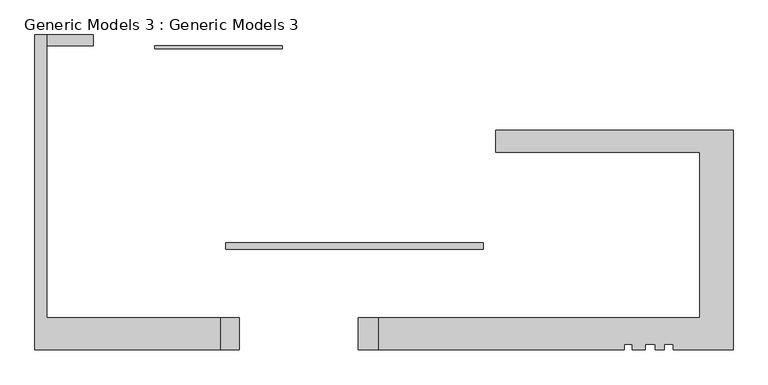
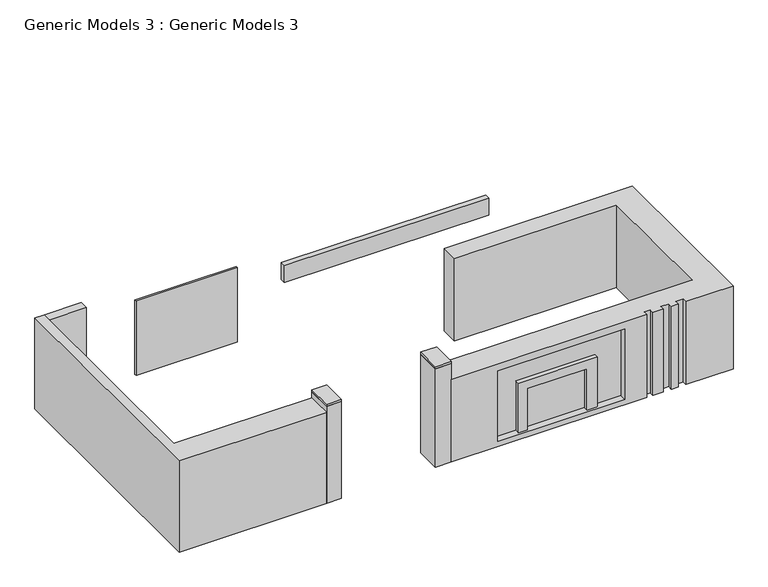
"""IFC4 building model written with IfcOpenShell, lengths in millimetres: proxy geometry, Generic Models 3 : Generic Models 3."""

from ifc_helpers import new_model, si_unit, frame, origin, origin_with_axes, place, context, project, spatial, polyline, outline, extrude, faceted_brep, source, transform, mapped, element, save


def generic_models_3_generic_models_3_20a2e421(model_context):
    return source(origin(), model_context, "Body", "SolidModel", [
        extrude(outline(polyline([(193.8418528, -5628.2321088), (193.8418528, -5323.4321088), (1717.8418528, -5323.4321088), (1717.8418528, -3243.1545541), (193.8418528, -3243.1545541), (193.8418528, -2885.0321088), (2022.6418528, -2885.0321088), (2022.6418528, -5628.2321088), (193.8418528, -5628.2321088)])), frame((0.0, -17714.7717874, 0.0), z_axis=(0.0, 1.0, 0.0), x_axis=(0.0, 0.0, 1.0)), (0.0, 0.0, 1.0), 152.4),
        extrude(outline(polyline([(-17488.9226696, -9095.6468404), (-17158.7226696, -9095.6468404), (-17158.7226696, -16906.1468404), (-12351.7136239, -16906.1468404), (-12351.7136239, -17790.9717874), (-17488.9226696, -17790.9717874), (-17488.9226696, -9095.6468404)])), origin_with_axes(), (0.0, 0.0, 1.0), 3352.8),
        faceted_brep([(886.8678912, -16906.1468404, 0.0), (886.8678912, -12332.3455275, 0.0), (-4751.9321088, -12332.3455275, 0.0), (-4751.9321088, -11722.7455275, 0.0), (1801.2678912, -11722.7455275, 0.0), (1801.2678912, -17790.9717874, 0.0), (149.2696895, -17790.9717874, 0.0), (149.2696895, -17638.5717874, 0.0), (-104.2990387, -17638.5717874, 0.0), (-104.2990387, -17790.9717874, 0.0), (-346.3419156, -17790.9717874, 0.0), (-346.3419156, -17638.5717874, 0.0), (-622.9623464, -17638.5717874, 0.0), (-622.9623464, -17790.9717874, 0.0), (-991.7895874, -17790.9717874, 0.0), (-991.7895874, -17638.5717874, 0.0), (-1205.7130534, -17638.5717874, 0.0), (-1205.7130534, -17790.9717874, 0.0), (-8007.6360274, -17790.9717874, 0.0), (-8007.6360274, -16906.1468404, 0.0), (886.8678912, -12332.3455275, 3048.0), (886.8678912, -16906.1468404, 3048.0), (-8007.6360274, -16906.1468404, 3048.0), (-8007.6360274, -17790.9717874, 3048.0), (-1205.7130534, -17790.9717874, 3048.0), (-1205.7130534, -17638.5717874, 3048.0), (-991.7895874, -17638.5717874, 3048.0), (-991.7895874, -17790.9717874, 3048.0), (-622.9623464, -17790.9717874, 3048.0), (-622.9623464, -17638.5717874, 3048.0), (-346.3419156, -17638.5717874, 3048.0), (-346.3419156, -17790.9717874, 3048.0), (-104.2990387, -17790.9717874, 3048.0), (-104.2990387, -17638.5717874, 3048.0), (149.2696895, -17638.5717874, 3048.0), (149.2696895, -17790.9717874, 3048.0), (1801.2678912, -17790.9717874, 3048.0), (1801.2678912, -11722.7455275, 3048.0), (-4751.9321088, -11722.7455275, 3048.0), (-4751.9321088, -12332.3455275, 3048.0), (-6394.384366, -17790.9717874, 193.8418528), (-6394.384366, -17790.9717874, 2784.6418528), (-1974.784366, -17790.9717874, 2784.6418528), (-1974.784366, -17790.9717874, 193.8418528), (-6394.384366, -17562.3717874, 193.8418528), (-1974.784366, -17562.3717874, 193.8418528), (-1974.784366, -17562.3717874, 2784.6418528), (-6394.384366, -17562.3717874, 2784.6418528)], [[[0, 1, 2, 3, 4, 5, 6, 7, 8, 9, 10, 11, 12, 13, 14, 15, 16, 17, 18, 19]], [[20, 21, 22, 23, 24, 25, 26, 27, 28, 29, 30, 31, 32, 33, 34, 35, 36, 37, 38, 39]], [[1, 0, 21, 20]], [[4, 37, 36, 5]], [[39, 2, 1, 20]], [[3, 2, 39, 38]], [[4, 3, 38, 37]], [[23, 18, 17, 24], [40, 41, 42, 43]], [[19, 22, 21, 0]], [[18, 23, 22, 19]], [[44, 45, 46, 47]], [[44, 47, 41, 40]], [[47, 46, 42, 41]], [[46, 45, 43, 42]], [[45, 44, 40, 43]], [[15, 26, 25, 16]], [[16, 25, 24, 17]], [[26, 15, 14, 27]], [[12, 29, 28, 13]], [[30, 11, 10, 31]], [[8, 33, 32, 9]], [[34, 7, 6, 35]], [[14, 13, 28, 27]], [[10, 9, 32, 31]], [[5, 36, 35, 6]], [[11, 30, 29, 12]], [[7, 34, 33, 8]]]),
        extrude(outline(polyline([(-17158.7226696, -9400.4468404), (-17158.7226696, -9095.6468404), (-15877.1321088, -9095.6468404), (-15877.1321088, -9400.4468404), (-17158.7226696, -9400.4468404)])), origin_with_axes(), (0.0, 0.0, 1.0), 3352.8),
        extrude(outline(polyline([(-12351.7136239, -16906.1468404), (-11844.8500069, -16906.1468404), (-11844.8500069, -17790.9717874), (-12351.7136239, -17790.9717874), (-12351.7136239, -16906.1468404)])), frame((0.0, 0.0, 3570.8534077), z_axis=(0.0, 0.0, 1.0), x_axis=(1.0, 0.0, 0.0)), (0.0, 0.0, 1.0), 76.2),
        extrude(outline(polyline([(-11844.8500069, -16906.1468404), (-11844.8500069, -17790.9717874), (-12351.7136239, -17790.9717874), (-12351.7136239, -16906.1468404), (-11844.8500069, -16906.1468404)])), origin_with_axes(), (0.0, 0.0, 1.0), 3570.8534077),
        extrude(outline(polyline([(-8561.9321088, -17790.9717874), (-8561.9321088, -16906.1468404), (-8007.6360274, -16906.1468404), (-8007.6360274, -17790.9717874), (-8561.9321088, -17790.9717874)])), frame((0.0, 0.0, 3627.9870628), z_axis=(0.0, 0.0, 1.0), x_axis=(1.0, 0.0, 0.0)), (0.0, 0.0, 1.0), 76.2),
        extrude(outline(polyline([(-8561.9321088, -17790.9717874), (-8561.9321088, -16906.1468404), (-8007.6360274, -16906.1468404), (-8007.6360274, -17790.9717874), (-8561.9321088, -17790.9717874)])), origin_with_axes(), (0.0, 0.0, 1.0), 3627.9870628),
        extrude(outline(polyline([(-10657.4321088, -9476.6468404), (-14180.7645284, -9476.6468404), (-14180.7645284, -9400.4468404), (-10657.4321088, -9400.4468404), (-10657.4321088, -9476.6468404)])), frame((0.0, 0.0, 304.8), z_axis=(0.0, 0.0, 1.0), x_axis=(1.0, 0.0, 0.0)), (0.0, 0.0, 1.0), 2743.2),
        faceted_brep([(-12215.152412, -14831.2402495, 7028.6159765), (-12215.152412, -15011.776778, 7028.6159765), (-5107.5321088, -15011.776778, 7028.6159765), (-5107.5321088, -14831.2402495, 7028.6159765), (-12215.152412, -14831.2402495, 6400.8), (-12128.9471301, -14831.2402495, 6400.8), (-5107.5321088, -14831.2402495, 6400.8), (-5107.5321088, -15011.776778, 6400.8), (-12215.152412, -15011.776778, 6400.8)], [[[0, 1, 2, 3]], [[4, 5, 6, 7, 8]], [[1, 0, 4, 8]], [[2, 1, 8, 7]], [[3, 2, 7, 6]], [[0, 3, 6, 5, 4]]]),
    ])


if __name__ == "__main__":
    model = new_model("IFC4")
    model_context = context("Model", 3, world=origin())
    ifc_project = project(units=[si_unit("LENGTHUNIT", "METRE", prefix="MILLI")], contexts=[model_context])
    site = spatial("IfcSite", under=ifc_project)
    building = spatial("IfcBuilding", under=site)
    placement = place(None, origin())
    generic_models_3_generic_models_3_shape = generic_models_3_generic_models_3_20a2e421(model_context)
    element("IfcBuildingElementProxy", 1, Name="Generic Models 3 : Generic Models 3", ObjectType="Generic Models 3 : Generic Models 3", at=placement, inside=building, context=model_context, shape_type="MappedRepresentation", body=[
        mapped(generic_models_3_generic_models_3_shape, transform((0.0, 0.0, 0.0), x_axis=(1.0, 0.0, 0.0), y_axis=(0.0, 1.0, 0.0), z_axis=(0.0, 0.0, 1.0))),
    ])
    save(model, "model.ifc")
